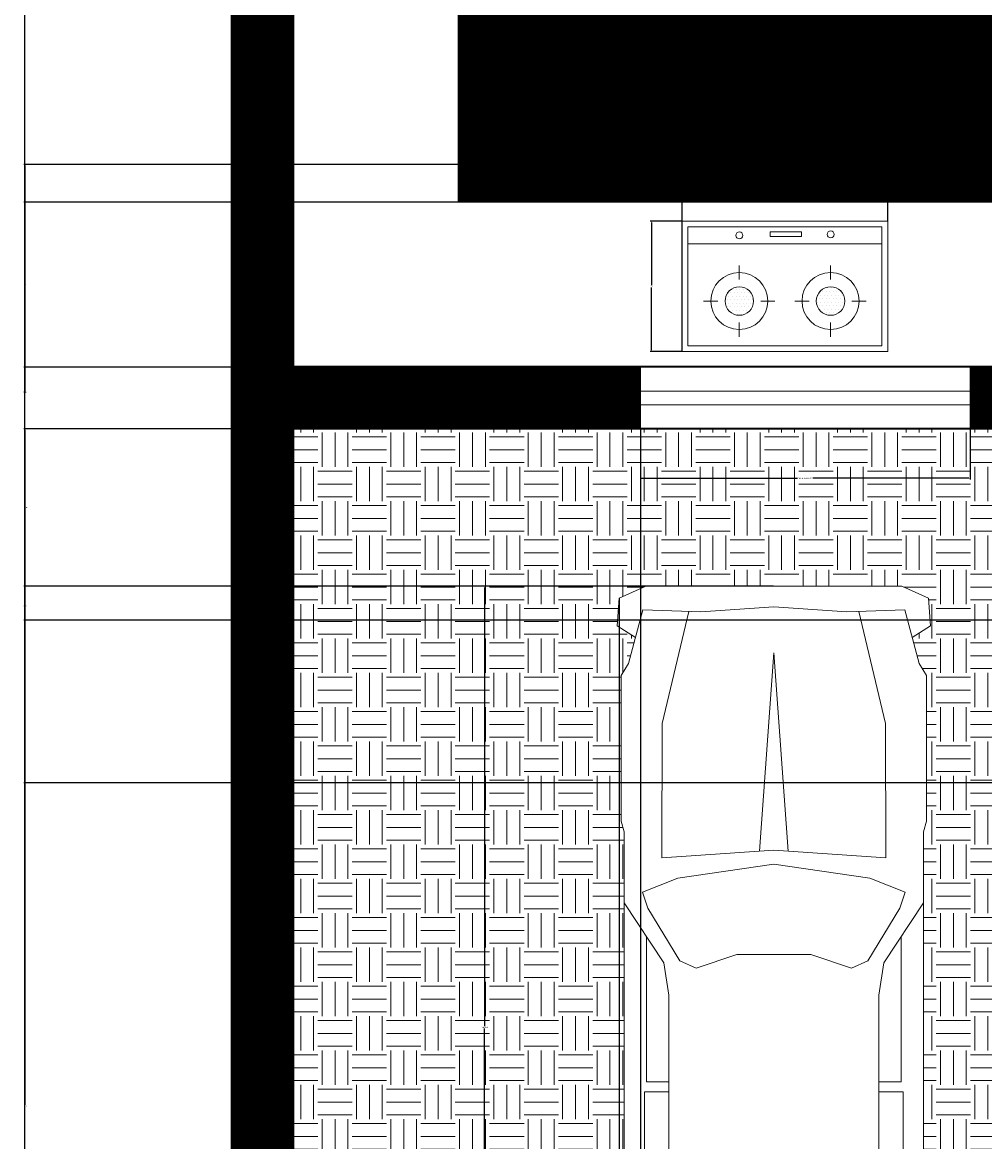
# Model space of a CAD drawing. Units: inches. Extents: x 205 to 1667, y -23 to 828.
# Tile 2 of 10: x 432 to 572, y 101 to 264. Entities that reach past the tile are written whole.
import ezdxf

# ---------------------------------------------------------------- set-up
doc = ezdxf.new("R2010")
doc.units = ezdxf.units.IN
doc.header["$MEASUREMENT"] = 0
for name, color, linetype, lineweight in [('A-ANNO-DIMS', 2, 'Continuous', 18), ('A-EQPM', 8, 'Continuous', 18), ('A-FLOR-CASE', 32, 'Continuous', 25), ('A-FLOR-PKNG', 8, 'Continuous', 18), ('A-GLAZ', 4, 'Continuous', 18), ('A-WALL', 7, 'Continuous', 35)]:
    doc.layers.add(name, color=color, linetype=linetype, lineweight=lineweight)
doc.layers.add('A-FLOR-PATT', color=9, linetype='Continuous', lineweight=9, true_color=0xc7c8ca)
doc.styles.get("Standard").update_dxf_attribs({"font": 'arial.ttf'})
doc.dimstyles.get("Standard").update_dxf_attribs({"dimtxt": 0.18, "dimasz": 0.18, "dimexe": 0.18, "dimexo": 0.0625, "dimgap": 0.09, "dimtad": 0, "dimtih": 1, "dimtoh": 1, "dimdec": 4, "dimzin": 0, "dimdsep": 46, "dimtxsty": 'Standard', "dimcen": 0.09, "dimadec": 0, "dimazin": 0, "dimtfac": 1, "dimtdec": 4, "dimtofl": 0, "dimtmove": 0, "dimatfit": 3, "dimfxl": 1, "dimtolj": 1, "dimtzin": 0, "dimarcsym": 0})

# ---------------------------------------------------------------- blocks, each defined once
blk = doc.blocks.new('A$C475E21CF')
for p, q in [((0, 444.5), (0, 0)), ((0, 444.5), (699.9, 444.5)), ((19.4, 425), (19.4, 19.4)), ((19.4, 425), (680.5, 425)), ((680.5, 425), (680.5, 19.4)), ((699.9, 444.5), (699.9, 0)), ((194.5, 393.9), (194.5, 345.2)), ((505.4, 393.9), (505.4, 345.2)), ((185.2, 312.7), (185.2, 312.7)), ((197.3, 312.7), (197.3, 312.7)), ((209.5, 312.7), (209.5, 312.7)), ((498.4, 316.6), (498.4, 316.6)), ((510.6, 316.6), (510.6, 316.6)), ((522.7, 316.6), (522.7, 316.6)), ((72.9, 272.3), (121.6, 272.3)), ((154.8, 276.2), (154.8, 276.2)), ((160.9, 288.4), (160.9, 288.4)), ((166.9, 300.5), (166.9, 300.5)), ((166.9, 276.2), (166.9, 276.2)), ((173, 288.4), (173, 288.4)), ((179.1, 300.5), (179.1, 300.5)), ((179.1, 276.2), (179.1, 276.2)), ((185.2, 288.4), (185.2, 288.4)), ((191.2, 300.5), (191.2, 300.5)), ((191.2, 276.2), (191.2, 276.2)), ((197.3, 288.4), (197.3, 288.4)), ((203.4, 300.5), (203.4, 300.5)), ((203.4, 276.2), (203.4, 276.2)), ((209.5, 288.4), (209.5, 288.4)), ((215.6, 300.5), (215.6, 300.5)), ((215.6, 276.2), (215.6, 276.2)), ((221.6, 288.4), (221.6, 288.4)), ((227.7, 300.5), (227.7, 300.5)), ((227.7, 276.2), (227.7, 276.2)), ((233.8, 288.4), (233.8, 288.4)), ((239.9, 276.2), (239.9, 276.2)), ((267.4, 272.3), (316, 272.3)), ((383.9, 272.3), (432.5, 272.3)), ((462, 268), (462, 268)), ((468, 280.2), (468, 280.2)), ((474.1, 292.3), (474.1, 292.3)), ((474.1, 268), (474.1, 268)), ((480.2, 304.5), (480.2, 304.5)), ((480.2, 280.2), (480.2, 280.2)), ((486.3, 292.3), (486.3, 292.3)), ((486.3, 268), (486.3, 268)), ((492.3, 304.5), (492.3, 304.5)), ((492.3, 280.2), (492.3, 280.2)), ((498.4, 292.3), (498.4, 292.3)), ((498.4, 268), (498.4, 268)), ((504.5, 304.5), (504.5, 304.5)), ((504.5, 280.2), (504.5, 280.2)), ((510.6, 292.3), (510.6, 292.3)), ((510.6, 268), (510.6, 268)), ((516.7, 304.5), (516.7, 304.5)), ((516.7, 280.2), (516.7, 280.2)), ((522.7, 292.3), (522.7, 292.3)), ((522.7, 268), (522.7, 268)), ((528.8, 304.5), (528.8, 304.5)), ((528.8, 280.2), (528.8, 280.2)), ((534.9, 292.3), (534.9, 292.3)), ((534.9, 268), (534.9, 268)), ((541, 304.5), (541, 304.5)), ((541, 280.2), (541, 280.2)), ((547, 292.3), (547, 292.3)), ((547, 268), (547, 268)), ((553.1, 280.2), (553.1, 280.2)), ((578.4, 272.3), (627, 272.3)), ((148.7, 264.1), (148.7, 264.1)), ((154.8, 251.9), (154.8, 251.9)), ((160.9, 264.1), (160.9, 264.1)), ((160.9, 239.8), (160.9, 239.8)), ((166.9, 251.9), (166.9, 251.9)), ((173, 264.1), (173, 264.1)), ((173, 239.8), (173, 239.8)), ((179.1, 251.9), (179.1, 251.9)), ((185.2, 264.1), (185.2, 264.1)), ((185.2, 239.8), (185.2, 239.8)), ((191.2, 251.9), (191.2, 251.9)), ((197.3, 264.1), (197.3, 264.1)), ((197.3, 239.8), (197.3, 239.8)), ((203.4, 251.9), (203.4, 251.9)), ((209.5, 264.1), (209.5, 264.1)), ((209.5, 239.8), (209.5, 239.8)), ((215.6, 251.9), (215.6, 251.9)), ((221.6, 264.1), (221.6, 264.1)), ((221.6, 239.8), (221.6, 239.8)), ((227.7, 251.9), (227.7, 251.9)), ((233.8, 264.1), (233.8, 264.1)), ((233.8, 239.8), (233.8, 239.8)), ((239.9, 251.9), (239.9, 251.9)), ((468, 255.9), (468, 255.9)), ((474.1, 243.7), (474.1, 243.7)), ((480.2, 255.9), (480.2, 255.9)), ((486.3, 243.7), (486.3, 243.7)), ((492.3, 255.9), (492.3, 255.9)), ((492.3, 231.5), (492.3, 231.5)), ((498.4, 243.7), (498.4, 243.7)), ((504.5, 255.9), (504.5, 255.9)), ((504.5, 231.5), (504.5, 231.5)), ((510.6, 243.7), (510.6, 243.7)), ((516.7, 255.9), (516.7, 255.9)), ((516.7, 231.5), (516.7, 231.5)), ((522.7, 243.7), (522.7, 243.7)), ((528.8, 255.9), (528.8, 255.9)), ((528.8, 231.5), (528.8, 231.5)), ((534.9, 243.7), (534.9, 243.7)), ((541, 255.9), (541, 255.9)), ((547, 243.7), (547, 243.7)), ((553.1, 255.9), (553.1, 255.9)), ((179.1, 227.6), (179.1, 227.6)), ((191.2, 227.6), (191.2, 227.6)), ((194.5, 199.4), (194.5, 150.8)), ((203.4, 227.6), (203.4, 227.6)), ((215.6, 227.6), (215.6, 227.6)), ((505.4, 199.4), (505.4, 150.8)), ((19.4, 77.8), (680.5, 77.8)), ((293.4, 51.9), (400.6, 51.9)), ((293.4, 36.5), (293.4, 51.9)), ((400.6, 51.9), (400.6, 36.5)), ((0, 0), (699.9, 0)), ((19.4, 19.4), (680.5, 19.4)), ((400.6, 36.5), (293.4, 36.5))]:
    blk.add_line(p, q)
for centre, radius in [((194.5, 272.3), 97.2), ((505.4, 272.3), 97.2), ((194.5, 272.3), 48.6), ((505.4, 272.3), 48.6), ((193.9, 45.1), 11.7), ((505.2, 48.5), 11.7)]:
    blk.add_circle(centre, radius)
blk = doc.blocks.new('A$C1A936BB7')
blk.add_blockref('A$C475E21CF', (0, 0))
blk = doc.blocks.new('A$C3BDD66A0')
for p, q in [((-1.5608, 0.7448), (-1.6934, 0.7345)), ((-1.5055, 0.6573), (-1.5608, 0.7448)), ((-1.6934, 0.7345), (-1.7501, 0.6077)), ((-1.383, 0.6896), (-1.3262, 0.7247)), ((-1.3262, 0.7247), (-0.6328, 0.7247)), ((-0.6328, 0.7247), (-0.5818, 0.7108)), ((-0.5818, 0.7108), (1.0338, 0.7108)), ((0.0405, 0.522), (-0.2453, 0.7108)), ((1.0338, 0.7108), (1.1052, 0.7328)), ((1.1052, 0.7328), (1.8759, 0.7328)), ((1.8759, 0.7328), (1.9021, 0.6971)), ((1.9021, 0.6971), (2.2838, 0.6931)), ((2.2533, 0.6934), (2.2838, 0.7237)), ((2.2838, 0.7237), (2.3654, 0.7238)), ((2.2838, 0.6931), (2.2999, 0.6319)), ((2.3654, 0.7238), (2.4427, 0.6569)), ((-1.6379, 0.6224), (-1.383, 0.6896)), ((2.4427, 0.6569), (2.4427, 0.3509)), ((-1.7501, 0.6077), (-1.7501, 0)), ((-1.6275, 0.3471), (-1.6379, 0.6224)), ((-0.363, 0.4561), (-0.2962, 0.6237)), ((-0.363, 0.4561), (-0.2962, 0.6237)), ((-0.2962, 0.6237), (-0.2204, 0.599)), ((-0.2962, 0.6237), (-0.2204, 0.599)), ((-0.2204, 0.599), (0.0303, 0.4462)), ((-0.2204, 0.599), (0.0303, 0.4462)), ((-0.0842, 0.6044), (0.6056, 0.6044)), ((0.6056, 0.6044), (0.6056, 0.499)), ((0.6523, 0.6144), (2.0654, 0.6144)), ((0.6523, 0.499), (0.6523, 0.6144)), ((2.0654, 0.6144), (2.2228, 0.5809)), ((2.2999, 0.6319), (2.3146, 0.5344)), ((2.2228, 0.5809), (2.3146, 0.5096)), ((2.3146, 0.5344), (2.3146, 0)), ((-1.6296, 0.403), (-1.0973, 0.5311)), ((-1.0973, 0.5311), (-0.4592, 0.5317)), ((-0.4592, 0.5317), (-0.4952, 0)), ((0.1935, 0.499), (0.0405, 0.522)), ((1.9475, 0.499), (0.1935, 0.499)), ((2.0903, 0.4482), (1.9475, 0.499)), ((-0.4282, 0), (-0.363, 0.4561)), ((-0.4282, 0), (-0.363, 0.4561)), ((0.0303, 0.4462), (0.0654, 0.3691)), ((0.0303, 0.4462), (0.0654, 0.3691)), ((2.1315, 0.3666), (2.0903, 0.4482)), ((2.1927, 0.3914), (2.2229, 0.4425)), ((2.2229, 0.4425), (2.2739, 0.4076)), ((2.1927, 0.0506), (2.1927, 0.3914)), ((2.2739, 0.4076), (2.2742, 0.0448)), ((-1.6519, 0), (-1.6275, 0.3471)), ((0.0654, 0.3691), (0, 0.1752)), ((0.0654, 0.3691), (0, 0.1752)), ((2.1315, 0), (2.1315, 0.3666)), ((2.4427, 0.3509), (2.3964, 0.3159)), ((2.3964, 0.3159), (2.3146, 0.3056)), ((0, 0.1752), (0, 0)), ((0, 0.1752), (0, 0)), ((-1.4334, 0), (-0.4906, 0.0678)), ((-1.7501, -0.6077), (-1.7501, 0)), ((-1.6519, 0), (-1.6275, -0.3471)), ((-1.4334, 0), (-0.4906, -0.0678)), ((-0.4592, -0.5317), (-0.4952, 0)), ((-0.4282, 0), (-0.363, -0.4561)), ((-0.4282, 0), (-0.363, -0.4561)), ((0, -0.1752), (0, 0)), ((0, -0.1752), (0, 0)), ((2.1315, 0), (2.1315, -0.3666)), ((2.3146, 0), (2.1315, 0)), ((2.2437, 0.0244), (2.1927, 0.0506)), ((2.2742, 0.0448), (2.2437, 0.0244)), ((2.3146, -0.5344), (2.3146, 0)), ((2.2437, -0.0244), (2.1927, -0.0506)), ((2.1927, -0.0506), (2.1927, -0.3914)), ((2.2742, -0.0448), (2.2437, -0.0244)), ((2.2739, -0.4076), (2.2742, -0.0448)), ((0.0654, -0.3691), (0, -0.1752)), ((0.0654, -0.3691), (0, -0.1752)), ((2.3964, -0.3159), (2.3146, -0.3056)), ((2.4427, -0.3509), (2.3964, -0.3159)), ((-1.6275, -0.3471), (-1.6379, -0.6224)), ((0.0303, -0.4462), (0.0654, -0.3691)), ((0.0303, -0.4462), (0.0654, -0.3691)), ((2.1315, -0.3666), (2.0903, -0.4482)), ((2.4427, -0.6569), (2.4427, -0.3509)), ((-1.6296, -0.403), (-1.0973, -0.5311)), ((2.1927, -0.3914), (2.2229, -0.4425)), ((2.2229, -0.4425), (2.2739, -0.4076)), ((-0.363, -0.4561), (-0.2962, -0.6237)), ((-0.363, -0.4561), (-0.2962, -0.6237)), ((-0.2204, -0.599), (0.0303, -0.4462)), ((-0.2204, -0.599), (0.0303, -0.4462)), ((2.0903, -0.4482), (1.9475, -0.499)), ((-1.0973, -0.5311), (-0.4592, -0.5317)), ((0.0405, -0.522), (-0.2453, -0.7108)), ((0.1935, -0.499), (0.0405, -0.522)), ((1.9475, -0.499), (0.1935, -0.499)), ((0.6056, -0.6044), (0.6056, -0.499)), ((0.6523, -0.499), (0.6523, -0.6144)), ((2.2228, -0.5809), (2.3146, -0.5096)), ((2.0654, -0.6144), (2.2228, -0.5809)), ((2.2999, -0.6319), (2.3146, -0.5344)), ((-1.6934, -0.7345), (-1.7501, -0.6077)), ((-1.6379, -0.6224), (-1.383, -0.6896)), ((-0.2962, -0.6237), (-0.2204, -0.599)), ((-0.2962, -0.6237), (-0.2204, -0.599)), ((-0.0842, -0.6044), (0.6056, -0.6044)), ((0.6523, -0.6144), (2.0654, -0.6144)), ((2.2838, -0.6931), (2.2999, -0.6319)), ((-1.5055, -0.6573), (-1.5608, -0.7448)), ((-1.383, -0.6896), (-1.3262, -0.7247)), ((2.3654, -0.7238), (2.4427, -0.6569)), ((-1.5608, -0.7448), (-1.6934, -0.7345)), ((-1.3262, -0.7247), (-0.6328, -0.7247)), ((-0.6328, -0.7247), (-0.5818, -0.7108)), ((-0.5818, -0.7108), (1.0338, -0.7108)), ((1.0338, -0.7108), (1.1052, -0.7328)), ((1.1052, -0.7328), (1.8759, -0.7328)), ((1.8759, -0.7328), (1.9021, -0.6971)), ((1.9021, -0.6971), (2.2838, -0.6931)), ((2.2533, -0.6934), (2.2838, -0.7237)), ((2.2838, -0.7237), (2.3654, -0.7238))]:
    blk.add_line(p, q)
blk = doc.blocks.new('WIN-48IN')
for p, q in [((0, 0), (0, 9)), ((0, 9), (48, 9)), ((48, 9), (48, 0)), ((48, 5.5), (0, 5.5)), ((48, 3.5), (0, 3.5)), ((48, 0), (0, 0))]:
    blk.add_line(p, q)
blk = doc.blocks.new('*D18')
at = {"layer": 'A-ANNO-DIMS', "color": 0, "lineweight": -2, "transparency": 16777216}
for p, q in [((521.94, 204.87), (521.94, 197.55)), ((569.94, 204.87), (569.94, 197.55)), ((522.12, 197.73), (544.82, 197.73)), ((569.76, 197.73), (547.05, 197.73))]:
    blk.add_line(p, q, dxfattribs=at)
at = {"layer": 'A-ANNO-DIMS', "color": 0, "transparency": 16777216}
for points in [[(522.12, 197.76), (522.12, 197.7), (521.94, 197.73)], [(569.76, 197.76), (569.76, 197.7), (569.94, 197.73)]]:
    blk.add_solid(points, dxfattribs=at)
at = {"layer": 'Defpoints', "color": 0, "transparency": 16777216}
for p in [(521.94, 204.93), (569.94, 204.93), (569.94, 197.73)]:
    blk.add_point(p, dxfattribs=at)
at = {"layer": 'A-ANNO-DIMS', "color": 0, "transparency": 16777216, "insert": (545.94, 197.73), "char_height": 0.18, "attachment_point": 5}
blk.add_mtext('\\A1;WINDOW 48 TYP.', dxfattribs=at)
blk = doc.blocks.new('*D19')
at = {"layer": 'A-ANNO-DIMS', "color": 0, "lineweight": -2, "transparency": 16777216}
for p, q in [((570, 213.93), (577.32, 213.93)), ((577.14, 213.75), (577.14, 209.61)), ((577.14, 205.11), (577.14, 209.25)), ((570, 204.93), (577.32, 204.93))]:
    blk.add_line(p, q, dxfattribs=at)
at = {"layer": 'A-ANNO-DIMS', "color": 0, "transparency": 16777216}
for points in [[(577.11, 213.75), (577.17, 213.75), (577.14, 213.93)], [(577.11, 205.11), (577.17, 205.11), (577.14, 204.93)]]:
    blk.add_solid(points, dxfattribs=at)
at = {"layer": 'Defpoints', "color": 0, "transparency": 16777216}
for p in [(569.94, 213.93), (577.14, 213.93), (569.94, 204.93)]:
    blk.add_point(p, dxfattribs=at)
at = {"layer": 'A-ANNO-DIMS', "color": 0, "transparency": 16777216, "insert": (577.14, 209.43), "char_height": 0.18, "attachment_point": 5}
blk.add_mtext('\\A1;9 TYP.', dxfattribs=at)
blk = doc.blocks.new('*D32')
at = {"layer": 'A-ANNO-DIMS', "color": 0, "lineweight": -2, "transparency": 16777216}
for p, q in [((528.03, 235.23), (528.03, 239.83)), ((528.21, 239.65), (542.1, 239.65)), ((557.76, 239.65), (543.86, 239.65)), ((557.94, 235.23), (557.94, 239.83))]:
    blk.add_line(p, q, dxfattribs=at)
at = {"layer": 'A-ANNO-DIMS', "color": 0, "transparency": 16777216}
for points in [[(528.21, 239.68), (528.21, 239.62), (528.03, 239.65)], [(557.76, 239.68), (557.76, 239.62), (557.94, 239.65)]]:
    blk.add_solid(points, dxfattribs=at)
at = {"layer": 'Defpoints', "color": 0, "transparency": 16777216}
for p in [(528.03, 239.65), (528.03, 235.17), (557.94, 235.17)]:
    blk.add_point(p, dxfattribs=at)
at = {"layer": 'A-ANNO-DIMS', "color": 0, "transparency": 16777216, "insert": (542.98, 239.65), "char_height": 0.18, "attachment_point": 5}
blk.add_mtext('\\A1;COOKTOP 30', dxfattribs=at)
blk = doc.blocks.new('*D33')
at = {"layer": 'A-ANNO-DIMS', "color": 0, "lineweight": -2, "transparency": 16777216}
for p, q in [((527.97, 235.17), (523.37, 235.17)), ((523.55, 234.99), (523.55, 225.86)), ((523.55, 216.36), (523.55, 225.49)), ((527.97, 216.18), (523.37, 216.18))]:
    blk.add_line(p, q, dxfattribs=at)
at = {"layer": 'A-ANNO-DIMS', "color": 0, "transparency": 16777216}
for points in [[(523.52, 234.99), (523.58, 234.99), (523.55, 235.17)], [(523.52, 216.36), (523.58, 216.36), (523.55, 216.18)]]:
    blk.add_solid(points, dxfattribs=at)
at = {"layer": 'Defpoints', "color": 0, "transparency": 16777216}
for p in [(528.03, 235.17), (523.55, 216.18), (528.03, 216.18)]:
    blk.add_point(p, dxfattribs=at)
at = {"layer": 'A-ANNO-DIMS', "color": 0, "transparency": 16777216, "insert": (523.55, 225.67), "char_height": 0.18, "attachment_point": 5}
blk.add_mtext('\\A1;19', dxfattribs=at)
blk = doc.blocks.new('*D40')
at = {"layer": 'A-ANNO-DIMS', "color": 0, "lineweight": -2, "transparency": 16777216}
for p, q in [((518.48, 182.02), (499.09, 182.02)), ((499.27, 181.84), (499.27, 117.96)), ((499.27, 53.72), (499.27, 117.59)), ((518.48, 53.54), (499.09, 53.54))]:
    blk.add_line(p, q, dxfattribs=at)
at = {"layer": 'A-ANNO-DIMS', "color": 0, "transparency": 16777216}
for points in [[(499.24, 181.84), (499.3, 181.84), (499.27, 182.02)], [(499.24, 53.72), (499.3, 53.72), (499.27, 53.54)]]:
    blk.add_solid(points, dxfattribs=at)
at = {"layer": 'Defpoints', "color": 0, "transparency": 16777216}
for p in [(518.54, 182.02), (499.27, 53.54), (518.54, 53.54)]:
    blk.add_point(p, dxfattribs=at)
at = {"layer": 'A-ANNO-DIMS', "color": 0, "transparency": 16777216, "insert": (499.27, 117.78), "char_height": 0.18, "attachment_point": 5}
blk.add_mtext('\\A1;CAR 128', dxfattribs=at)
blk = doc.blocks.new('*D43')
at = {"layer": 'A-ANNO-DIMS', "color": 0, "lineweight": -2, "transparency": 16777216}
for p, q in [((462.37, 607.65), (432.19, 607.65)), ((432.37, 607.47), (432.37, 307.83)), ((432.37, 7.83), (432.37, 307.47)), ((462.37, 7.65), (432.19, 7.65))]:
    blk.add_line(p, q, dxfattribs=at)
at = {"layer": 'A-ANNO-DIMS', "color": 0, "transparency": 16777216}
for points in [[(432.34, 607.47), (432.4, 607.47), (432.37, 607.65)], [(432.34, 7.83), (432.4, 7.83), (432.37, 7.65)]]:
    blk.add_solid(points, dxfattribs=at)
at = {"layer": 'Defpoints', "color": 0, "transparency": 16777216}
for p in [(432.37, 607.65), (462.43, 607.65), (462.43, 7.65)]:
    blk.add_point(p, dxfattribs=at)
at = {"layer": 'A-ANNO-DIMS', "color": 0, "transparency": 16777216, "insert": (432.37, 307.65), "char_height": 0.18, "attachment_point": 5}
blk.add_mtext('\\A1;600', dxfattribs=at)
blk = doc.blocks.new('*D52')
at = {"layer": 'A-ANNO-DIMS', "color": 0, "lineweight": -2, "transparency": 16777216}
for p, q in [((471.43, 204.87), (471.43, -22.59)), ((521.94, 204.87), (521.94, -22.59)), ((471.61, -22.41), (496.36, -22.41)), ((521.76, -22.41), (497.01, -22.41))]:
    blk.add_line(p, q, dxfattribs=at)
at = {"layer": 'A-ANNO-DIMS', "color": 0, "transparency": 16777216}
for points in [[(471.61, -22.38), (471.61, -22.44), (471.43, -22.41)], [(521.76, -22.38), (521.76, -22.44), (521.94, -22.41)]]:
    blk.add_solid(points, dxfattribs=at)
at = {"layer": 'Defpoints', "color": 0, "transparency": 16777216}
for p in [(471.43, 204.93), (521.94, 204.93), (521.94, -22.41)]:
    blk.add_point(p, dxfattribs=at)
at = {"layer": 'A-ANNO-DIMS', "color": 0, "transparency": 16777216, "insert": (496.68, -22.41), "char_height": 0.18, "attachment_point": 5}
blk.add_mtext('\\A1;50.5', dxfattribs=at)
blk = doc.blocks.new('*D64')
at = {"layer": 'A-ANNO-DIMS', "color": 0, "lineweight": -2, "transparency": 16777216}
for p, q in [((471.43, 454.59), (471.43, -22.59)), ((583.44, 454.59), (583.44, -22.59)), ((471.61, -22.41), (527.16, -22.41)), ((583.26, -22.41), (527.71, -22.41))]:
    blk.add_line(p, q, dxfattribs=at)
at = {"layer": 'A-ANNO-DIMS', "color": 0, "transparency": 16777216}
for points in [[(471.61, -22.38), (471.61, -22.44), (471.43, -22.41)], [(583.26, -22.38), (583.26, -22.44), (583.44, -22.41)]]:
    blk.add_solid(points, dxfattribs=at)
at = {"layer": 'Defpoints', "color": 0, "transparency": 16777216}
for p in [(471.43, 454.65), (583.44, 454.65), (583.44, -22.41)]:
    blk.add_point(p, dxfattribs=at)
at = {"layer": 'A-ANNO-DIMS', "color": 0, "transparency": 16777216, "insert": (527.44, -22.41), "char_height": 0.18, "attachment_point": 5}
blk.add_mtext('\\A1;112', dxfattribs=at)
blk = doc.blocks.new('*D65')
at = {"layer": 'A-ANNO-DIMS', "color": 0, "lineweight": -2, "transparency": 16777216}
for p, q in [((617.28, 204.93), (432.19, 204.93)), ((432.37, 204.75), (432.37, 179.34)), ((432.37, 153.56), (432.37, 178.97)), ((617.28, 153.38), (432.19, 153.38))]:
    blk.add_line(p, q, dxfattribs=at)
at = {"layer": 'A-ANNO-DIMS', "color": 0, "transparency": 16777216}
for points in [[(432.34, 204.75), (432.4, 204.75), (432.37, 204.93)], [(432.34, 153.56), (432.4, 153.56), (432.37, 153.38)]]:
    blk.add_solid(points, dxfattribs=at)
at = {"layer": 'Defpoints', "color": 0, "transparency": 16777216}
for p in [(432.37, 204.93), (617.35, 204.93), (617.35, 153.38)]:
    blk.add_point(p, dxfattribs=at)
at = {"layer": 'A-ANNO-DIMS', "color": 0, "transparency": 16777216, "insert": (432.37, 179.15), "char_height": 0.18, "attachment_point": 5}
blk.add_mtext('\\A1;51.56', dxfattribs=at)
blk = doc.blocks.new('*D67')
at = {"layer": 'A-ANNO-DIMS', "color": 0, "lineweight": -2, "transparency": 16777216}
for p, q in [((691.44, 243.44), (432.19, 243.44)), ((432.37, 243.26), (432.37, 210.43)), ((432.37, 177.23), (432.37, 210.06)), ((691.44, 177.05), (432.19, 177.05))]:
    blk.add_line(p, q, dxfattribs=at)
at = {"layer": 'A-ANNO-DIMS', "color": 0, "transparency": 16777216}
for points in [[(432.34, 243.26), (432.4, 243.26), (432.37, 243.44)], [(432.34, 177.23), (432.4, 177.23), (432.37, 177.05)]]:
    blk.add_solid(points, dxfattribs=at)
at = {"layer": 'Defpoints', "color": 0, "transparency": 16777216}
for p in [(432.37, 243.44), (691.51, 243.44), (691.51, 177.05)]:
    blk.add_point(p, dxfattribs=at)
at = {"layer": 'A-ANNO-DIMS', "color": 0, "transparency": 16777216, "insert": (432.37, 210.24), "char_height": 0.18, "attachment_point": 5}
blk.add_mtext('\\A1;66.39', dxfattribs=at)
blk = doc.blocks.new('*D76')
at = {"layer": 'A-ANNO-DIMS', "color": 0, "lineweight": -2, "transparency": 16777216}
for p, q in [((471.43, 213.99), (471.43, 637.89)), ((471.61, 637.71), (499.41, 637.71)), ((527.85, 637.71), (500.05, 637.71)), ((528.03, 216.24), (528.03, 637.89))]:
    blk.add_line(p, q, dxfattribs=at)
at = {"layer": 'A-ANNO-DIMS', "color": 0, "transparency": 16777216}
for points in [[(471.61, 637.74), (471.61, 637.68), (471.43, 637.71)], [(527.85, 637.74), (527.85, 637.68), (528.03, 637.71)]]:
    blk.add_solid(points, dxfattribs=at)
at = {"layer": 'Defpoints', "color": 0, "transparency": 16777216}
for p in [(528.03, 637.71), (528.03, 216.18), (471.43, 213.93)]:
    blk.add_point(p, dxfattribs=at)
at = {"layer": 'A-ANNO-DIMS', "color": 0, "transparency": 16777216, "insert": (499.73, 637.71), "char_height": 0.18, "attachment_point": 5}
blk.add_mtext('\\A1;56.6', dxfattribs=at)
blk = doc.blocks.new('*D81')
at = {"layer": 'A-ANNO-DIMS', "color": 0, "lineweight": -2, "transparency": 16777216}
for p, q in [((596.38, 237.93), (432.19, 237.93)), ((432.37, 237.75), (432.37, 226.11)), ((432.37, 214.11), (432.37, 225.75)), ((596.38, 213.93), (432.19, 213.93))]:
    blk.add_line(p, q, dxfattribs=at)
at = {"layer": 'A-ANNO-DIMS', "color": 0, "transparency": 16777216}
for points in [[(432.34, 237.75), (432.4, 237.75), (432.37, 237.93)], [(432.34, 214.11), (432.4, 214.11), (432.37, 213.93)]]:
    blk.add_solid(points, dxfattribs=at)
at = {"layer": 'Defpoints', "color": 0, "transparency": 16777216}
for p in [(432.37, 237.93), (596.44, 237.93), (596.44, 213.93)]:
    blk.add_point(p, dxfattribs=at)
at = {"layer": 'A-ANNO-DIMS', "color": 0, "transparency": 16777216, "insert": (432.37, 225.93), "char_height": 0.18, "attachment_point": 5}
blk.add_mtext('\\A1;24', dxfattribs=at)
blk = doc.blocks.new('*D82')
at = {"layer": 'A-ANNO-DIMS', "color": 0, "lineweight": -2, "transparency": 16777216}
for p, q in [((471.43, 204.87), (471.43, -22.59)), ((518.86, 180.22), (518.86, -22.59)), ((471.61, -22.41), (494.75, -22.41)), ((518.68, -22.41), (495.54, -22.41))]:
    blk.add_line(p, q, dxfattribs=at)
at = {"layer": 'A-ANNO-DIMS', "color": 0, "transparency": 16777216}
for points in [[(471.61, -22.38), (471.61, -22.44), (471.43, -22.41)], [(518.68, -22.38), (518.68, -22.44), (518.86, -22.41)]]:
    blk.add_solid(points, dxfattribs=at)
at = {"layer": 'Defpoints', "color": 0, "transparency": 16777216}
for p in [(471.43, 204.93), (518.86, 180.28), (518.86, -22.41)]:
    blk.add_point(p, dxfattribs=at)
at = {"layer": 'A-ANNO-DIMS', "color": 0, "transparency": 16777216, "insert": (495.14, -22.41), "char_height": 0.18, "attachment_point": 5}
blk.add_mtext('\\A1;47.43', dxfattribs=at)
blk = doc.blocks.new('*D83')
at = {"layer": 'A-ANNO-DIMS', "color": 0, "lineweight": -2, "transparency": 16777216}
for p, q in [((471.37, 204.93), (432.19, 204.93)), ((432.37, 204.75), (432.37, 193.66)), ((432.37, 182.2), (432.37, 193.29)), ((541.3, 182.02), (432.19, 182.02))]:
    blk.add_line(p, q, dxfattribs=at)
at = {"layer": 'A-ANNO-DIMS', "color": 0, "transparency": 16777216}
for points in [[(432.34, 204.75), (432.4, 204.75), (432.37, 204.93)], [(432.34, 182.2), (432.4, 182.2), (432.37, 182.02)]]:
    blk.add_solid(points, dxfattribs=at)
at = {"layer": 'Defpoints', "color": 0, "transparency": 16777216}
for p in [(471.43, 204.93), (432.37, 182.02), (541.37, 182.02)]:
    blk.add_point(p, dxfattribs=at)
at = {"layer": 'A-ANNO-DIMS', "color": 0, "transparency": 16777216, "insert": (432.37, 193.47), "char_height": 0.18, "attachment_point": 5}
blk.add_mtext('\\A1;22.916', dxfattribs=at)
blk = doc.blocks.new('*D84')
at = {"layer": 'A-ANNO-DIMS', "color": 0, "lineweight": -2, "transparency": 16777216}
for p, q in [((471.37, 204.93), (432.19, 204.93)), ((432.37, 204.75), (432.37, 106.47)), ((432.37, 7.83), (432.37, 106.11)), ((471.37, 7.65), (432.19, 7.65))]:
    blk.add_line(p, q, dxfattribs=at)
at = {"layer": 'A-ANNO-DIMS', "color": 0, "transparency": 16777216}
for points in [[(432.34, 204.75), (432.4, 204.75), (432.37, 204.93)], [(432.34, 7.83), (432.4, 7.83), (432.37, 7.65)]]:
    blk.add_solid(points, dxfattribs=at)
at = {"layer": 'Defpoints', "color": 0, "transparency": 16777216}
for p in [(432.37, 204.93), (471.43, 204.93), (471.43, 7.65)]:
    blk.add_point(p, dxfattribs=at)
at = {"layer": 'A-ANNO-DIMS', "color": 0, "transparency": 16777216, "insert": (432.37, 106.29), "char_height": 0.18, "attachment_point": 5}
blk.add_mtext('\\A1;197.3', dxfattribs=at)

msp = doc.modelspace()

# ---------------------------------------------------------------- hatches: boundary and pattern name
at = {"layer": 'A-FLOR-PATT'}
h = msp.add_hatch(dxfattribs=at)
h.set_pattern_fill('ANSI31', color=256)
h.paths.add_polyline_path([(774.4305, 607.6511), (720.5338, 607.6511), (720.5338, 598.6511), (727.9933, 598.6511), (746.8614, 598.6511), (765.4305, 598.6511), (765.4305, 454.6511), (759.5298, 454.6511), (759.5298, 448.9635), (765.4305, 448.9635), (765.4305, 428.0602), (774.4305, 428.0602)])
h.paths.add_polyline_path([(765.4305, 598.6511), (746.8614, 598.6511), (746.8614, 579.7829), (727.9933, 579.7829), (727.9933, 518.1387, -0.41421701), (724.6389, 514.7843), (668.2693, 514.7843, -0.41421356), (665.0743, 517.9793), (665.0743, 579.7829), (646.2062, 579.7829), (646.2062, 598.6511), (626.3468, 598.6511), (626.3468, 454.6511), (628.3468, 454.6511), (628.3468, 484.9635, -0.41421356), (664.3468, 449.9635), (664.3468, 454.6511), (729.3305, 454.6511), (758.5298, 454.6511), (759.5298, 454.6511), (765.4305, 454.6511)])
h.paths.add_polyline_path([(621.4404, 598.6511), (471.4305, 598.6511), (471.4305, 568.8442), (490.2987, 568.8442), (490.2987, 549.9761), (551.9429, 549.9761, -0.41421701), (555.2973, 546.6217), (555.2973, 490.2521, -0.41421356), (552.1023, 487.0571), (490.2987, 487.0571), (490.2987, 468.189), (471.4305, 468.189), (471.4305, 454.6511), (583.4404, 454.6511), (583.4404, 449.9635, -0.41421356), (619.4404, 484.9635), (619.4404, 454.6511), (621.4404, 454.6511)])
h.paths.add_polyline_path([(672.5338, 607.6511), (569.5707, 607.6511), (569.5707, 598.6511), (621.4404, 598.6511), (621.4404, 454.6511), (619.4404, 454.6511), (619.4404, 448.9635), (628.3468, 448.9635), (628.3468, 454.6511), (626.3468, 454.6511), (626.3468, 598.6511), (646.2062, 598.6511), (665.0743, 598.6511), (672.5338, 598.6511)])
h.paths.add_polyline_path([(521.5707, 607.6511), (462.4305, 607.6511), (462.4305, 407.4306), (471.4305, 407.4306), (471.4305, 448.9635), (583.4404, 448.9635, -0.0070419), (583.4404, 449.9635), (583.4404, 454.6511), (471.4305, 454.6511), (471.4305, 468.189), (471.4305, 487.0571), (471.4305, 549.9761), (471.4305, 568.8442), (471.4305, 598.6511), (521.5707, 598.6511)])
h.paths.add_polyline_path([(471.4305, 314.3187), (583.4404, 314.3187), (583.4404, 319.9388), (471.4305, 319.9388), (471.4305, 359.4306), (462.4305, 359.4306), (462.4305, 7.6511), (471.4305, 7.6511), (471.4305, 204.9321), (521.9355, 204.9321), (521.9355, 213.9321), (471.4305, 213.9321)])
h.paths.add_polyline_path([(774.4305, 410.0602), (765.4305, 410.0602), (765.4305, 389.1569), (672.3024, 389.1569), (672.3024, 448.9635), (681.1739, 448.9635, -0.18532444), (681.6564, 449.1487), (698.6035, 449.1487), (729.3305, 448.9635), (729.3305, 454.6511), (664.3468, 454.6511), (664.3468, 449.9635, -0.0070419), (664.3468, 448.9635), (666.3024, 448.9635), (666.3024, 378.2485), (672.3024, 378.2485), (672.3024, 383.1306), (765.4305, 383.1306), (765.4305, 360.5347), (774.4305, 360.5347)])
h.paths.add_polyline_path([(774.4305, 342.5347), (765.4305, 342.5347), (765.4305, 319.9388), (672.3024, 319.9388), (672.3024, 348.5574), (671.0896, 348.5574, -0.04071533), (666.3024, 348.2485), (666.3024, 319.9388), (664.3468, 319.9388, -0.0070419), (664.3468, 318.9388), (664.3468, 314.3187), (765.4305, 314.3187), (765.4305, 290.8426), (774.4305, 290.8426)])
h.paths.add_polyline_path([(774.4305, 242.8426), (765.4305, 242.8426), (765.4305, 104.6382), (626.3468, 104.6382), (626.3468, 110.5917), (617.3468, 110.5917), (617.3468, 95.6382), (765.4305, 95.6382), (765.4305, 16.6511), (621.2232, 16.6511), (621.2232, 7.6511), (774.4305, 7.6511)])
h.paths.add_polyline_path([(626.3468, 314.3187), (628.3468, 314.3187), (628.3468, 319.9388), (619.4404, 319.9388), (619.4404, 314.3187), (620.4404, 314.3187), (620.4404, 213.9321), (569.9355, 213.9321), (569.9355, 204.9321), (617.3468, 204.9321), (617.3468, 153.3751), (626.3468, 153.3751)])
h.paths.add_polyline_path([(620.4404, 314.3187), (619.4404, 314.3187), (619.4404, 319.9388), (628.3468, 319.9388), (629.3468, 319.9388), (629.3468, 283.9388, 0.40598745), (664.3468, 318.9388), (664.3468, 319.9388), (666.3024, 319.9388), (666.3024, 348.2485), (666.3024, 377.2485), (666.3024, 378.2485), (666.3024, 448.9635), (664.3468, 448.9635), (664.3468, 449.9635, 0.40598745), (629.3468, 484.9635), (629.3468, 448.9635), (628.3468, 448.9635), (619.4404, 448.9635), (618.4404, 448.9635), (618.4404, 484.9635, 0.40598745), (583.4404, 449.9635), (583.4404, 448.9635), (471.4305, 448.9635), (471.4305, 407.4306), (471.4305, 359.4306), (471.4305, 319.9388), (583.4404, 319.9388), (583.4404, 314.3187), (495.4305, 314.3187), (495.4305, 237.9321), (620.4404, 237.9321)])
h.paths.add_polyline_path([(525.0876, 347.7863), (513.5657, 347.7863), (512.0216, 362.1672), (526.6317, 362.1672)], flags=16)
h.paths.add_polyline_path([(550.9499, 370.1471), (536.569, 368.6029), (536.569, 383.2131), (550.9499, 381.6689)], flags=16)
h.paths.add_polyline_path([(530.7713, 364.5431), (508.0415, 364.5431, -0.41421356), (504.7944, 367.7902), (504.7944, 403.5085, -0.41421356), (508.0415, 406.7556), (530.7713, 406.7556, -0.41421356), (534.0184, 403.5085), (534.0184, 367.7902, -0.41421356)], flags=16)
h.paths.add_polyline_path([(550.9499, 389.6298), (536.569, 388.0856), (536.569, 402.6958), (550.9499, 401.1516)], flags=16)
h.paths.add_polyline_path([(502.2439, 368.6029), (487.863, 370.1471), (487.863, 381.6689), (502.2439, 383.2131)], flags=16)
h.paths.add_polyline_path([(502.2439, 388.0856), (487.863, 389.6298), (487.863, 401.1516), (502.2439, 402.6958)], flags=16)
h.paths.add_polyline_path([(526.6317, 409.1315), (512.0216, 409.1315), (513.5657, 423.5124), (525.0876, 423.5124)], flags=16)
h.paths.add_polyline_path([(765.4305, 290.8426), (765.4305, 314.3187), (664.3468, 314.3187), (664.3468, 318.9388, -0.41421356), (628.3468, 283.9388), (628.3468, 314.3187), (626.3468, 314.3187), (626.3468, 153.3751), (638.3468, 153.3751, -0.4196361), (617.5748, 131.9834, -0.4196361), (638.3468, 110.5917), (626.3468, 110.5917), (626.3468, 104.6382), (765.4305, 104.6382), (765.4305, 242.8426)])
h.paths.add_polyline_path([(691.5064, 243.4363), (693.2483, 243.4363), (725.4984, 243.4363), (725.4984, 241.7329), (725.4984, 177.0512), (723.7564, 177.0512), (691.5064, 177.0512), (691.5064, 178.7545)], flags=16)
h.paths.add_polyline_path([(689.8658, 265.2977), (689.8658, 296.6873, -0.41421356), (690.8346, 297.6561), (724.6111, 297.6561, -0.41421356), (725.5799, 296.6873), (725.5799, 265.2977, -0.41421356), (724.6111, 264.3289), (690.8346, 264.3289, -0.41421356)], flags=16)
h.paths.add_polyline_path([(694.1286, 265.6852), (694.1286, 288.9368, -0.41421356), (695.0974, 289.9056), (720.3483, 289.9056, -0.41421356), (721.3171, 288.9368), (721.3171, 265.6852, -0.04533947), (721.3013, 265.5106, -0.3531705), (720.3282, 264.7164), (695.0974, 264.7164, -0.41421356)], flags=0)
h.paths.add_polyline_path([(694.1286, 291.2619), (694.1286, 294.7497, -0.41421356), (695.0974, 295.7185), (720.3483, 295.7185, -0.41421356), (721.3171, 294.7497), (721.3171, 291.2619, -0.41421356), (720.3483, 290.2931), (695.0974, 290.2931, -0.41421356)], flags=0)
h.paths.add_polyline_path([(734.4369, 244.6615, -0.41421356), (735.2682, 245.4928), (762.2019, 245.4928, -0.41421356), (763.0332, 244.6615), (763.0332, 168.183, -0.41421356), (762.2019, 167.3517), (735.2682, 167.3517, -0.41421356), (734.4369, 168.183)], flags=16)
h.paths.add_polyline_path([(761.7032, 242.1676), (761.7032, 170.6768), (735.6007, 171.0093, -0.41421356), (734.7694, 171.8406), (734.7694, 193.5102, -0.56972741), (735.6007, 194.674, -0.41421356), (734.7694, 195.5053), (734.7694, 217.3423, -0.56972741), (735.6007, 218.5061, -0.41421356), (734.7694, 219.3374), (734.7694, 241.0038, -0.41421356), (735.6007, 241.8351), (735.1643, 242.1676)], flags=16)
h.paths.add_polyline_path([(757.5467, 171.0093), (760.5393, 171.0093, 0.41421356), (761.3706, 171.8406), (761.3706, 193.5102, 0.41421356), (760.5393, 194.3415), (757.5467, 194.3415, 0.41421356), (756.7154, 193.5102), (756.7155, 171.8534, 0.41871477)], flags=0)
h.paths.add_polyline_path([(756.7154, 241.0038, -0.41421356), (757.5467, 241.8351), (760.5393, 241.8351, -0.41421356), (761.3706, 241.0038), (761.3706, 219.3374, -0.41421356), (760.5393, 218.5061), (760.5393, 218.1736, -0.41421356), (761.3706, 217.3423), (761.3706, 195.5053, -0.41421356), (760.5393, 194.674), (757.5467, 194.674, -0.56972741), (756.3829, 195.5053, -0.41421356), (755.5516, 194.674), (755.5516, 194.3415, -0.41421356), (756.3829, 193.5102), (756.7154, 171.8406), (756.3829, 193.5102, 0.41421356), (755.5516, 194.3415), (735.6007, 194.674), (755.5516, 194.674, 0.41421356), (756.3829, 195.5053), (756.3829, 217.3423, 0.41421356), (755.5516, 218.1736), (735.6007, 218.5061), (755.5516, 218.5061, 0.41421356), (756.3829, 219.3374)], flags=0)
h.paths.add_polyline_path([(694.5151, 150.3608), (728.2916, 150.3608, -0.41421356), (729.2604, 149.3919), (729.2604, 118.0023, -0.41421356), (728.2916, 117.0335), (694.5151, 117.0335, -0.41421356), (693.5463, 118.0023), (693.5463, 149.3919, -0.41421356)], flags=16)
h.paths.add_polyline_path([(724.0288, 149.9732, -0.41421356), (724.9977, 149.0044), (724.9977, 125.7529, -0.41421356), (724.0288, 124.784), (698.7779, 124.784, -0.41421356), (697.8091, 125.7529), (697.8091, 149.0044, -0.04533947), (697.825, 149.179, -0.3531705), (698.798, 149.9732)], flags=0)
h.paths.add_polyline_path([(698.7779, 124.3965), (724.0288, 124.3965, -0.41421356), (724.9977, 123.4277), (724.9977, 119.94, -0.41421356), (724.0288, 118.9711), (698.7779, 118.9711, -0.41421356), (697.8091, 119.94), (697.8091, 123.4277, -0.41421356)], flags=0)
h = msp.add_hatch(dxfattribs=at)
h.set_pattern_fill('EARTH', color=256, scale=20)
h.paths.add_polyline_path([(617.3468, 204.9321), (471.4305, 204.9321), (471.4305, 7.6511), (621.2232, 7.6511), (621.2232, 95.6382), (617.3468, 95.6382), (617.3468, 110.5917), (617.3468, 111.5917)])
h.paths.add_polyline_path([(564.1913, 176.2169), (561.5098, 174.5217), (562.5, 170.769), (563.5731, 169.029), (563.5731, 147.7805), (563.1483, 146.2164), (563.1483, 96.7087), (563.8223, 94.5214), (563.8223, 70.9058), (562.7294, 70.1011), (562.6164, 59.3401), (563.5441, 58.4056), (563.5465, 55.9057), (561.4952, 53.5377), (552.1213, 53.5377), (551.0475, 54.9563), (550.7331, 57.4626), (541.3672, 57.4626), (532.0012, 57.4626), (531.6868, 54.9563), (530.613, 53.5377), (521.2392, 53.5377), (519.1879, 55.9057), (519.1903, 58.4056), (520.1179, 59.3401), (520.0049, 70.1011), (518.912, 70.9058), (518.912, 94.5214), (519.5861, 96.7087), (519.5861, 146.2164), (519.1613, 147.7805), (519.1613, 169.029), (520.2343, 170.769), (521.2245, 174.5217), (518.5431, 176.2169), (518.8594, 180.2791), (522.745, 182.0164), (541.3672, 182.0164), (559.9894, 182.0164), (563.8749, 180.2791)], flags=16)
h.paths.add_polyline_path([(553.7175, 178.3241), (557.6423, 162.0145), (557.6609, 142.4613), (541.3672, 143.5621), (525.0735, 142.4613), (525.092, 162.0145), (529.0169, 178.3241), (530.7323, 178.2589), (541.3672, 179.0078), (552.002, 178.2589)], flags=0)
h.paths.add_polyline_path([(560.4781, 137.464), (559.7214, 135.1419), (555.0412, 127.459), (552.6762, 126.3854), (546.7369, 128.3886), (541.3672, 128.3886), (535.9975, 128.3886), (530.0582, 126.3854), (527.6931, 127.459), (523.013, 135.1419), (522.2563, 137.464), (527.3921, 139.5127), (541.3672, 141.5088), (555.3423, 139.5127)], flags=0)
h.paths.add_polyline_path([(559.8869, 130.9684), (559.8869, 109.832), (556.6594, 109.832), (556.6594, 68.7114), (555.1011, 64.335), (552.6025, 63.0718), (541.3672, 63.0718), (530.1319, 63.0718), (527.6333, 64.335), (526.075, 68.7114), (526.075, 109.832), (522.8474, 109.832), (522.8474, 130.9684), (525.3715, 127.1487), (526.075, 122.4588), (526.075, 68.7114), (527.6333, 64.335), (530.1319, 63.0718), (541.3672, 63.0718), (552.6025, 63.0718), (555.1011, 64.335), (556.6594, 68.7114), (556.6594, 122.4588), (557.3629, 127.1487)], flags=0)
h.paths.add_polyline_path([(553.3621, 61.1985), (554.9264, 60.2724), (553.8564, 58.7089), (542.7405, 58.6984), (542.1147, 59.6353), (542.9167, 61.1985)], flags=0)
h.paths.add_polyline_path([(539.8176, 61.1985), (540.6197, 59.6353), (539.9938, 58.6984), (528.8779, 58.7089), (527.808, 60.2724), (529.3722, 61.1985)], flags=0)

# ---------------------------------------------------------------- linework, layer by layer
at = {"layer": 'A-FLOR-CASE'}
for p in [(495.4305, 314.3187), (620.4404, 237.9321)]:
    msp.add_line(p, (495.4305, 237.9321), dxfattribs=at)
at = {"layer": 'A-WALL'}
for p, q in [((462.4305, 607.6511), (462.4305, 7.6511)), ((471.4305, 314.3187), (471.4305, 213.9321)), ((620.4404, 213.9321), (471.4305, 213.9321)), ((471.4305, 204.9321), (471.4305, 7.6511)), ((617.3468, 204.9321), (471.4305, 204.9321))]:
    msp.add_line(p, q, dxfattribs=at)

# ---------------------------------------------------------------- block references
at = {"layer": 'A-EQPM', "xscale": 0.0427250111418614, "yscale": 0.0427250111418614, "zscale": 0.0427250111418614, "rotation": 180}
msp.add_blockref('A$C1A936BB7', (557.9355, 235.1692), dxfattribs=at)
at = {"layer": 'A-FLOR-PKNG', "xscale": 30.6431746435358, "yscale": 30.6431746435358, "zscale": 30.6431746435358, "rotation": 270}
msp.add_blockref('A$C3BDD66A0', (541.3672, 128.3886), dxfattribs=at)
at = {"layer": 'A-GLAZ'}
msp.add_blockref('WIN-48IN', (521.9357, 204.932), dxfattribs=at)

# ---------------------------------------------------------------- dimensions: what is measured, and where the dimension line sits
at = {"layer": 'A-ANNO-DIMS'}
for base, p1, p2, override, picture, middle in [((528.0312, 637.7086), (471.4305, 213.9321), (528.0312, 216.1782), {"dimdec": 1, "dimlfac": 1, "dimrnd": 0, "dimzin": 0, "dimdsep": 46, "dimlunit": 2}, '*D76', (499.7309, 637.7086)), ((583.4404, -22.4064), (471.4305, 454.6511), (583.4404, 454.6511), {"dimdec": 0, "dimlfac": 1, "dimrnd": 0, "dimzin": 0, "dimdsep": 46, "dimlunit": 2}, '*D64', (527.4355, -22.4064)), ((521.9355, -22.4064), (471.4305, 204.9321), (521.9355, 204.9321), {"dimdec": 1, "dimlfac": 1, "dimrnd": 0, "dimzin": 0, "dimdsep": 46, "dimlunit": 2}, '*D52', (496.683, -22.4064)), ((518.8594, -22.4064), (471.4305, 204.9321), (518.8594, 180.2791), {"dimdec": 2, "dimlfac": 1, "dimrnd": 0, "dimzin": 0, "dimdsep": 46, "dimlunit": 2}, '*D82', (495.145, -22.4064))]:
    dim = msp.add_linear_dim(base=base, p1=p1, p2=p2, dimstyle='Standard', override=override, dxfattribs=at)
    dim.commit()
    dim.dimension.update_dxf_attribs({"geometry": picture, "text_midpoint": middle})
for base, p1, p2, angle, override, picture, middle in [((432.3731, 607.6511), (462.4305, 7.6511), (462.4305, 607.6511), 90, {"dimdec": 0, "dimlfac": 1, "dimrnd": 0, "dimzin": 0, "dimdsep": 46, "dimlunit": 2}, '*D43', (432.3731, 307.6511)), ((432.3731, 243.4363), (691.5064, 177.0512), (691.5064, 243.4363), 90, {"dimdec": 2, "dimlfac": 1, "dimrnd": 0, "dimzin": 0, "dimdsep": 46, "dimlunit": 2}, '*D67', (432.3731, 210.2437)), ((432.3731, 237.9321), (596.4404, 213.9321), (596.4404, 237.9321), 90, {"dimdec": 0, "dimlfac": 1, "dimrnd": 0, "dimzin": 0, "dimdsep": 46, "dimlunit": 2}, '*D81', (432.3731, 225.9321)), ((523.5456, 216.1782), (528.0312, 235.1692), (528.0312, 216.1782), 270, {"dimdec": 0, "dimlfac": 1, "dimrnd": 0, "dimzin": 0, "dimdsep": 46, "dimlunit": 2}, '*D33', (523.5456, 225.6737)), ((432.3731, 182.0164), (471.4305, 204.9321), (541.3672, 182.0164), 90, {"dimdec": 3, "dimlfac": 1, "dimrnd": 0, "dimzin": 0, "dimdsep": 46, "dimlunit": 2}, '*D83', (432.3731, 193.4743)), ((432.3731, 204.9321), (617.3468, 153.3751), (617.3468, 204.9321), 90, {"dimdec": 2, "dimlfac": 1, "dimrnd": 0, "dimzin": 0, "dimdsep": 46, "dimlunit": 2}, '*D65', (432.3731, 179.1536)), ((432.3731, 204.9321), (471.4305, 7.6511), (471.4305, 204.9321), 90, {"dimdec": 1, "dimlfac": 1, "dimrnd": 0, "dimzin": 0, "dimdsep": 46, "dimlunit": 2}, '*D84', (432.3731, 106.2916))]:
    dim = msp.add_linear_dim(base=base, p1=p1, p2=p2, angle=angle, dimstyle='Standard', override=override, dxfattribs=at)
    dim.commit()
    dim.dimension.update_dxf_attribs({"geometry": picture, "text_midpoint": middle})
for base, p1, p2, angle, text, picture, middle in [((528.0312, 239.6548), (557.9355, 235.1692), (528.0312, 235.1692), 180, 'COOKTOP <>', '*D32', (542.9833, 239.6548)), ((577.1355, 213.9321), (569.9355, 204.9321), (569.9355, 213.9321), 90, '<> TYP.', '*D19', (577.1355, 209.4321)), ((499.2713, 53.5377), (518.5431, 182.0164), (518.5431, 53.5377), 270, 'CAR <>', '*D40', (499.2713, 117.7771))]:
    dim = msp.add_linear_dim(base=base, p1=p1, p2=p2, angle=angle, text=text, dimstyle='Standard', override={"dimdec": 0, "dimlfac": 1, "dimrnd": 0, "dimzin": 0, "dimdsep": 46, "dimlunit": 2}, dxfattribs=at)
    dim.commit()
    dim.dimension.update_dxf_attribs({"geometry": picture, "text_midpoint": middle})
dim = msp.add_linear_dim(base=(569.9355, 197.7321), p1=(521.9355, 204.9321), p2=(569.9355, 204.9321), text='WINDOW <> TYP.', dimstyle='Standard', override={"dimdec": 0, "dimlfac": 1, "dimrnd": 0, "dimzin": 0, "dimdsep": 46, "dimlunit": 2}, dxfattribs=at)
dim.commit()
dim.dimension.update_dxf_attribs({"geometry": '*D18', "text_midpoint": (545.9355, 197.7321)})

doc.saveas('drawing.dxf')
